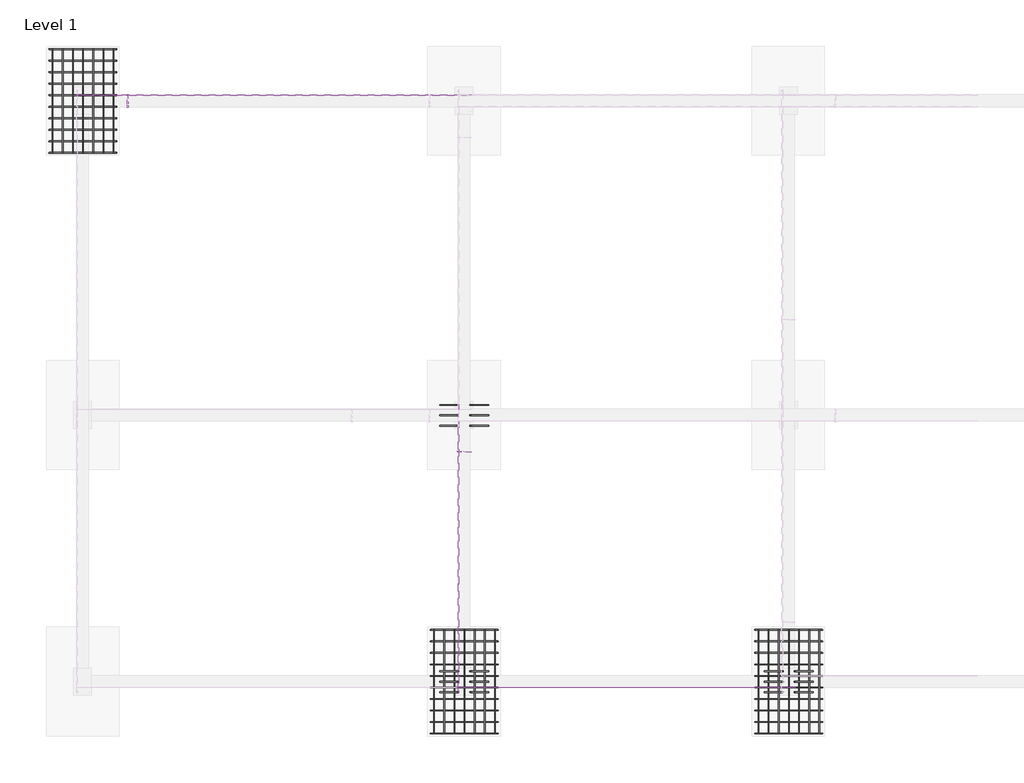
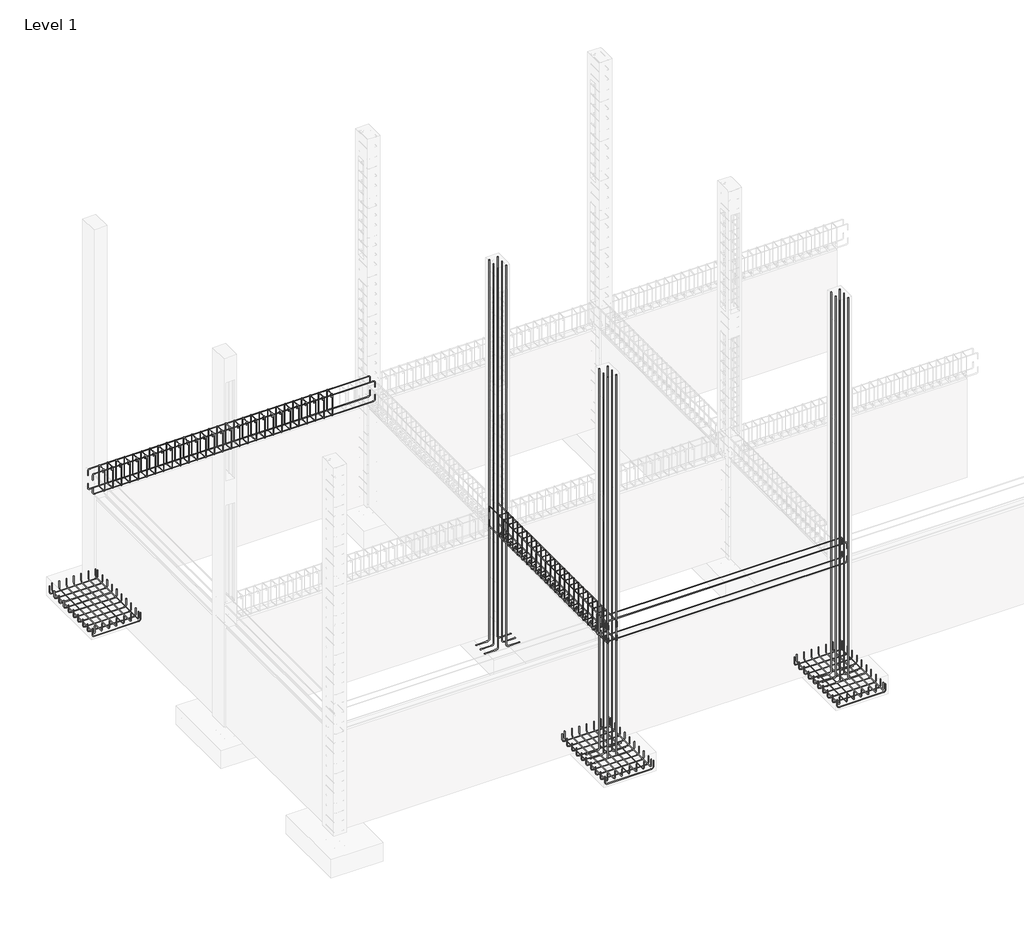
# One storey, part 4 of 8: 20 reinforcing bars.
"""IFC4 building model written with IfcOpenShell, lengths in millimetres."""

from ifc_helpers import new_model, si_unit, point, frame, origin, place, context, project, spatial, polyline, circle_curve, trimmed, segment, composite_curve, source, transform, mapped, element, save
from ifc_brep_helpers import swept_disk

model = new_model("IFC4")

# Units and contexts
model_context = context("Model", 3, world=origin())
ifc_project = project(units=[si_unit("LENGTHUNIT", "METRE", prefix="MILLI")], contexts=[model_context])

# Site, building, storey
site = spatial("IfcSite", under=ifc_project)
building = spatial("IfcBuilding", under=site)
storey = spatial("IfcBuildingStorey", under=building, Name="Level 1", Elevation=0.0)

# Reinforcing bars
placement = place(None, origin())
reinforcing_bar_shape = source(origin(), model_context, "Body", "SolidModel", [
    swept_disk(composite_curve([segment(polyline([(-8807.3422157, 3219.1306965, 2643.0183362), (-8807.3422157, 3219.1306965, 2528.7183362)]), True, "CONTINUOUS"), segment(trimmed(circle_curve(frame((-8841.8862157, 3219.1306965, 2528.7183362), z_axis=(0.0, 1.0, 0.0), x_axis=(34.54399999999987, 0.0, 0.0)), 34.544), [point((-8807.3422157, 3219.1306965, 2528.7183362))], [point((-8841.8862157, 3219.1306965, 2494.1743362))], True, "CARTESIAN"), True, "CONTINUOUS"), segment(polyline([(-8841.8862157, 3219.1306965, 2494.1743362), (-14435.2471545, 3219.1306965, 2494.1743362)]), True, "CONTINUOUS"), segment(trimmed(circle_curve(frame((-14435.2471545, 3219.1306965, 2528.7183362), z_axis=(0.0, 1.0, 0.0), x_axis=(0.0, 0.0, -34.54399999999987)), 34.544), [point((-14435.2471545, 3219.1306965, 2494.1743362))], [point((-14469.7911545, 3219.1306965, 2528.7183362))], True, "CARTESIAN"), True, "CONTINUOUS"), segment(polyline([(-14469.7911545, 3219.1306965, 2528.7183362), (-14469.7911545, 3219.1306965, 2643.0183362)]), True, "CONTINUOUS")], self_intersect=False), 5.969),
])
element("IfcReinforcingBar", 1, at=placement, inside=storey, context=model_context, shape_type="MappedRepresentation", body=[
    mapped(reinforcing_bar_shape, transform((0.0, 0.0, 0.0), x_axis=(1.0, 0.0, 0.0), y_axis=(0.0, 1.0, 0.0), z_axis=(0.0, 0.0, 1.0))),
    mapped(reinforcing_bar_shape, transform((0.0, -193.2513276, 0.0), x_axis=(1.0, 0.0, 0.0), y_axis=(0.0, 1.0, 0.0), z_axis=(0.0, 0.0, 1.0))),
])
reinforcing_bar_2_shape = source(origin(), model_context, "Body", "SolidModel", [
    swept_disk(composite_curve([segment(polyline([(-14469.7911545, 3219.1306965, 2843.3816638), (-14469.7911545, 3219.1306965, 2957.6816638)]), True, "CONTINUOUS"), segment(trimmed(circle_curve(frame((-14435.2471545, 3219.1306965, 2957.6816638), z_axis=(0.0, 1.0, 0.0), x_axis=(-34.54399999999987, 0.0, 0.0)), 34.544), [point((-14469.7911545, 3219.1306965, 2957.6816638))], [point((-14435.2471545, 3219.1306965, 2992.2256638))], True, "CARTESIAN"), True, "CONTINUOUS"), segment(polyline([(-14435.2471545, 3219.1306965, 2992.2256638), (-8841.8862157, 3219.1306965, 2992.2256638)]), True, "CONTINUOUS"), segment(trimmed(circle_curve(frame((-8841.8862157, 3219.1306965, 2957.6816638), z_axis=(0.0, 1.0, 0.0), x_axis=(0.0, 0.0, 34.54399999999987)), 34.544), [point((-8841.8862157, 3219.1306965, 2992.2256638))], [point((-8807.3422157, 3219.1306965, 2957.6816638))], True, "CARTESIAN"), True, "CONTINUOUS"), segment(polyline([(-8807.3422157, 3219.1306965, 2957.6816638), (-8807.3422157, 3219.1306965, 2843.3816638)]), True, "CONTINUOUS")], self_intersect=False), 5.969),
])
element("IfcReinforcingBar", 2, at=placement, inside=storey, context=model_context, shape_type="MappedRepresentation", body=[
    mapped(reinforcing_bar_2_shape, transform((0.0, 0.0, 0.0), x_axis=(1.0, 0.0, 0.0), y_axis=(0.0, 1.0, 0.0), z_axis=(0.0, 0.0, 1.0))),
    mapped(reinforcing_bar_2_shape, transform((0.0, -193.2513276, 0.0), x_axis=(1.0, 0.0, 0.0), y_axis=(0.0, 1.0, 0.0), z_axis=(0.0, 0.0, 1.0))),
])
reinforcing_bar_3_shape = source(origin(), model_context, "Body", "SolidModel", [
    swept_disk(composite_curve([segment(polyline([(-14263.0351545, 7767.9070829, 9105.9), (-14263.0351545, 7767.9070829, -307.9115)]), True, "CONTINUOUS"), segment(trimmed(circle_curve(frame((-14216.9341545, 7767.9070829, -307.9115), z_axis=(0.0, -1.0, 0.0), x_axis=(-46.10099999999875, 0.0, 0.0)), 46.101), [point((-14263.0351545, 7767.9070829, -307.9115))], [point((-14216.9341545, 7767.9070829, -354.0125))], True, "CARTESIAN"), True, "CONTINUOUS"), segment(polyline([(-14216.9341545, 7767.9070829, -354.0125), (-13950.3611545, 7767.9070829, -354.0125)]), True, "CONTINUOUS")], self_intersect=False), 8.001),
])
element("IfcReinforcingBar", 3, at=placement, inside=storey, context=model_context, shape_type="MappedRepresentation", body=[
    mapped(reinforcing_bar_3_shape, transform((0.0, 0.0, 0.0), x_axis=(1.0, 0.0, 0.0), y_axis=(0.0, 1.0, 0.0), z_axis=(0.0, 0.0, 1.0))),
    mapped(reinforcing_bar_3_shape, transform((0.0, -174.625, 0.0), x_axis=(1.0, 0.0, 0.0), y_axis=(0.0, 1.0, 0.0), z_axis=(0.0, 0.0, 1.0))),
    mapped(reinforcing_bar_3_shape, transform((0.0, -349.25, 0.0), x_axis=(1.0, 0.0, 0.0), y_axis=(0.0, 1.0, 0.0), z_axis=(0.0, 0.0, 1.0))),
])
reinforcing_bar_4_shape = source(origin(), model_context, "Body", "SolidModel", [
    swept_disk(composite_curve([segment(polyline([(-14772.5591545, 7767.9070829, -354.0125), (-14505.9861545, 7767.9070829, -354.0125)]), True, "CONTINUOUS"), segment(trimmed(circle_curve(frame((-14505.9861545, 7767.9070829, -307.9115), z_axis=(0.0, -1.0, 0.0), x_axis=(0.0, 0.0, -46.101)), 46.101), [point((-14505.9861545, 7767.9070829, -354.0125))], [point((-14459.8851545, 7767.9070829, -307.9115))], True, "CARTESIAN"), True, "CONTINUOUS"), segment(polyline([(-14459.8851545, 7767.9070829, -307.9115), (-14459.8851545, 7767.9070829, 9105.9)]), True, "CONTINUOUS")], self_intersect=False), 8.001),
])
element("IfcReinforcingBar", 4, at=placement, inside=storey, context=model_context, shape_type="MappedRepresentation", body=[
    mapped(reinforcing_bar_4_shape, transform((0.0, 0.0, 0.0), x_axis=(1.0, 0.0, 0.0), y_axis=(0.0, 1.0, 0.0), z_axis=(0.0, 0.0, 1.0))),
    mapped(reinforcing_bar_4_shape, transform((0.0, -174.625, 0.0), x_axis=(1.0, 0.0, 0.0), y_axis=(0.0, 1.0, 0.0), z_axis=(0.0, 0.0, 1.0))),
    mapped(reinforcing_bar_4_shape, transform((0.0, -349.25, 0.0), x_axis=(1.0, 0.0, 0.0), y_axis=(0.0, 1.0, 0.0), z_axis=(0.0, 0.0, 1.0))),
])
reinforcing_bar_5_shape = source(origin(), model_context, "Body", "SolidModel", [
    swept_disk(composite_curve([segment(polyline([(-14263.0351545, 3297.1300327, 9105.9), (-14263.0351545, 3297.1300327, -307.9115)]), True, "CONTINUOUS"), segment(trimmed(circle_curve(frame((-14216.9341545, 3297.1300327, -307.9115), z_axis=(0.0, -1.0, 0.0), x_axis=(-46.10099999999875, 0.0, 0.0)), 46.101), [point((-14263.0351545, 3297.1300327, -307.9115))], [point((-14216.9341545, 3297.1300327, -354.0125))], True, "CARTESIAN"), True, "CONTINUOUS"), segment(polyline([(-14216.9341545, 3297.1300327, -354.0125), (-13950.3611545, 3297.1300327, -354.0125)]), True, "CONTINUOUS")], self_intersect=False), 8.001),
])
element("IfcReinforcingBar", 5, at=placement, inside=storey, context=model_context, shape_type="MappedRepresentation", body=[
    mapped(reinforcing_bar_5_shape, transform((0.0, 0.0, 0.0), x_axis=(1.0, 0.0, 0.0), y_axis=(0.0, 1.0, 0.0), z_axis=(0.0, 0.0, 1.0))),
    mapped(reinforcing_bar_5_shape, transform((0.0, -174.625, 0.0), x_axis=(1.0, 0.0, 0.0), y_axis=(0.0, 1.0, 0.0), z_axis=(0.0, 0.0, 1.0))),
    mapped(reinforcing_bar_5_shape, transform((0.0, -349.25, 0.0), x_axis=(1.0, 0.0, 0.0), y_axis=(0.0, 1.0, 0.0), z_axis=(0.0, 0.0, 1.0))),
])
reinforcing_bar_6_shape = source(origin(), model_context, "Body", "SolidModel", [
    swept_disk(composite_curve([segment(polyline([(-14772.5591545, 3297.1300327, -354.0125), (-14505.9861545, 3297.1300327, -354.0125)]), True, "CONTINUOUS"), segment(trimmed(circle_curve(frame((-14505.9861545, 3297.1300327, -307.9115), z_axis=(0.0, -1.0, 0.0), x_axis=(0.0, 0.0, -46.101)), 46.101), [point((-14505.9861545, 3297.1300327, -354.0125))], [point((-14459.8851545, 3297.1300327, -307.9115))], True, "CARTESIAN"), True, "CONTINUOUS"), segment(polyline([(-14459.8851545, 3297.1300327, -307.9115), (-14459.8851545, 3297.1300327, 9105.9)]), True, "CONTINUOUS")], self_intersect=False), 8.001),
])
element("IfcReinforcingBar", 6, at=placement, inside=storey, context=model_context, shape_type="MappedRepresentation", body=[
    mapped(reinforcing_bar_6_shape, transform((0.0, 0.0, 0.0), x_axis=(1.0, 0.0, 0.0), y_axis=(0.0, 1.0, 0.0), z_axis=(0.0, 0.0, 1.0))),
    mapped(reinforcing_bar_6_shape, transform((0.0, -174.625, 0.0), x_axis=(1.0, 0.0, 0.0), y_axis=(0.0, 1.0, 0.0), z_axis=(0.0, 0.0, 1.0))),
    mapped(reinforcing_bar_6_shape, transform((0.0, -349.25, 0.0), x_axis=(1.0, 0.0, 0.0), y_axis=(0.0, 1.0, 0.0), z_axis=(0.0, 0.0, 1.0))),
])
reinforcing_bar_7_shape = source(origin(), model_context, "Body", "SolidModel", [
    swept_disk(composite_curve([segment(polyline([(-8817.2482157, 3297.1300327, 9105.9), (-8817.2482157, 3297.1300327, -307.9115)]), True, "CONTINUOUS"), segment(trimmed(circle_curve(frame((-8771.1472157, 3297.1300327, -307.9115), z_axis=(0.0, -1.0, 0.0), x_axis=(-46.10099999999875, 0.0, 0.0)), 46.101), [point((-8817.2482157, 3297.1300327, -307.9115))], [point((-8771.1472157, 3297.1300327, -354.0125))], True, "CARTESIAN"), True, "CONTINUOUS"), segment(polyline([(-8771.1472157, 3297.1300327, -354.0125), (-8504.5742157, 3297.1300327, -354.0125)]), True, "CONTINUOUS")], self_intersect=False), 8.001),
])
element("IfcReinforcingBar", 7, at=placement, inside=storey, context=model_context, shape_type="MappedRepresentation", body=[
    mapped(reinforcing_bar_7_shape, transform((0.0, 0.0, 0.0), x_axis=(1.0, 0.0, 0.0), y_axis=(0.0, 1.0, 0.0), z_axis=(0.0, 0.0, 1.0))),
    mapped(reinforcing_bar_7_shape, transform((0.0, -174.625, 0.0), x_axis=(1.0, 0.0, 0.0), y_axis=(0.0, 1.0, 0.0), z_axis=(0.0, 0.0, 1.0))),
    mapped(reinforcing_bar_7_shape, transform((0.0, -349.25, 0.0), x_axis=(1.0, 0.0, 0.0), y_axis=(0.0, 1.0, 0.0), z_axis=(0.0, 0.0, 1.0))),
])
reinforcing_bar_8_shape = source(origin(), model_context, "Body", "SolidModel", [
    swept_disk(composite_curve([segment(polyline([(-9326.7722157, 3297.1300327, -354.0125), (-9060.1992157, 3297.1300327, -354.0125)]), True, "CONTINUOUS"), segment(trimmed(circle_curve(frame((-9060.1992157, 3297.1300327, -307.9115), z_axis=(0.0, -1.0, 0.0), x_axis=(0.0, 0.0, -46.101)), 46.101), [point((-9060.1992157, 3297.1300327, -354.0125))], [point((-9014.0982157, 3297.1300327, -307.9115))], True, "CARTESIAN"), True, "CONTINUOUS"), segment(polyline([(-9014.0982157, 3297.1300327, -307.9115), (-9014.0982157, 3297.1300327, 9105.9)]), True, "CONTINUOUS")], self_intersect=False), 8.001),
])
element("IfcReinforcingBar", 8, at=placement, inside=storey, context=model_context, shape_type="MappedRepresentation", body=[
    mapped(reinforcing_bar_8_shape, transform((0.0, 0.0, 0.0), x_axis=(1.0, 0.0, 0.0), y_axis=(0.0, 1.0, 0.0), z_axis=(0.0, 0.0, 1.0))),
    mapped(reinforcing_bar_8_shape, transform((0.0, -174.625, 0.0), x_axis=(1.0, 0.0, 0.0), y_axis=(0.0, 1.0, 0.0), z_axis=(0.0, 0.0, 1.0))),
    mapped(reinforcing_bar_8_shape, transform((0.0, -349.25, 0.0), x_axis=(1.0, 0.0, 0.0), y_axis=(0.0, 1.0, 0.0), z_axis=(0.0, 0.0, 1.0))),
])
reinforcing_bar_9_shape = source(origin(), model_context, "Body", "SolidModel", [
    swept_disk(composite_curve([segment(polyline([(-20200.6033089, 13741.9865262, -216.662), (-20200.6033089, 13741.9865262, -369.062)]), True, "CONTINUOUS"), segment(trimmed(circle_curve(frame((-20244.6723089, 13741.9865262, -369.062), z_axis=(0.0, 1.0, 0.0), x_axis=(44.068999999999505, 0.0, 0.0)), 44.069), [point((-20200.6033089, 13741.9865262, -369.062))], [point((-20244.6723089, 13741.9865262, -413.131))], True, "CARTESIAN"), True, "CONTINUOUS"), segment(polyline([(-20244.6723089, 13741.9865262, -413.131), (-21287.5963089, 13741.9865262, -413.131)]), True, "CONTINUOUS"), segment(trimmed(circle_curve(frame((-21287.5963089, 13741.9865262, -369.062), z_axis=(0.0, 1.0, 0.0), x_axis=(0.0, 0.0, -44.06899999999996)), 44.069), [point((-21287.5963089, 13741.9865262, -413.131))], [point((-21331.6653089, 13741.9865262, -369.062))], True, "CARTESIAN"), True, "CONTINUOUS"), segment(polyline([(-21331.6653089, 13741.9865262, -369.062), (-21331.6653089, 13741.9865262, -216.662)]), True, "CONTINUOUS")], self_intersect=False), 5.969),
])
element("IfcReinforcingBar", 9, at=placement, inside=storey, context=model_context, shape_type="MappedRepresentation", body=[
    mapped(reinforcing_bar_9_shape, transform((0.0, 0.0, 0.0), x_axis=(1.0, 0.0, 0.0), y_axis=(0.0, 1.0, 0.0), z_axis=(0.0, 0.0, 1.0))),
    mapped(reinforcing_bar_9_shape, transform((0.0, -193.4068889, 0.0), x_axis=(1.0, 0.0, 0.0), y_axis=(0.0, 1.0, 0.0), z_axis=(0.0, 0.0, 1.0))),
    mapped(reinforcing_bar_9_shape, transform((0.0, -386.8137778, 0.0), x_axis=(1.0, 0.0, 0.0), y_axis=(0.0, 1.0, 0.0), z_axis=(0.0, 0.0, 1.0))),
    mapped(reinforcing_bar_9_shape, transform((0.0, -580.2206667, 0.0), x_axis=(1.0, 0.0, 0.0), y_axis=(0.0, 1.0, 0.0), z_axis=(0.0, 0.0, 1.0))),
    mapped(reinforcing_bar_9_shape, transform((0.0, -773.6275556, 0.0), x_axis=(1.0, 0.0, 0.0), y_axis=(0.0, 1.0, 0.0), z_axis=(0.0, 0.0, 1.0))),
    mapped(reinforcing_bar_9_shape, transform((0.0, -967.0344444, 0.0), x_axis=(1.0, 0.0, 0.0), y_axis=(0.0, 1.0, 0.0), z_axis=(0.0, 0.0, 1.0))),
    mapped(reinforcing_bar_9_shape, transform((0.0, -1160.4413333, 0.0), x_axis=(1.0, 0.0, 0.0), y_axis=(0.0, 1.0, 0.0), z_axis=(0.0, 0.0, 1.0))),
    mapped(reinforcing_bar_9_shape, transform((0.0, -1353.8482222, 0.0), x_axis=(1.0, 0.0, 0.0), y_axis=(0.0, 1.0, 0.0), z_axis=(0.0, 0.0, 1.0))),
    mapped(reinforcing_bar_9_shape, transform((0.0, -1547.2551111, 0.0), x_axis=(1.0, 0.0, 0.0), y_axis=(0.0, 1.0, 0.0), z_axis=(0.0, 0.0, 1.0))),
    mapped(reinforcing_bar_9_shape, transform((0.0, -1740.662, 0.0), x_axis=(1.0, 0.0, 0.0), y_axis=(0.0, 1.0, 0.0), z_axis=(0.0, 0.0, 1.0))),
])
reinforcing_bar_10_shape = source(origin(), model_context, "Body", "SolidModel", [
    swept_disk(composite_curve([segment(polyline([(-21274.1343089, 13741.9865262, -165.481), (-21274.1343089, 13741.9865262, -317.881)]), True, "CONTINUOUS"), segment(trimmed(circle_curve(frame((-21274.1343089, 13697.9175262, -317.881), z_axis=(-1.0, 0.0, 0.0), x_axis=(0.0, 44.068999999999505, 0.0)), 44.069), [point((-21274.1343089, 13741.9865262, -317.881))], [point((-21274.1343089, 13697.9175262, -361.95))], True, "CARTESIAN"), True, "CONTINUOUS"), segment(polyline([(-21274.1343089, 13697.9175262, -361.95), (-21274.1343089, 12045.3935262, -361.95)]), True, "CONTINUOUS"), segment(trimmed(circle_curve(frame((-21274.1343089, 12045.3935262, -317.881), z_axis=(-1.0, 0.0, 0.0), x_axis=(0.0, 0.0, -44.06900000000002)), 44.069), [point((-21274.1343089, 12045.3935262, -361.95))], [point((-21274.1343089, 12001.3245262, -317.881))], True, "CARTESIAN"), True, "CONTINUOUS"), segment(polyline([(-21274.1343089, 12001.3245262, -317.881), (-21274.1343089, 12001.3245262, -165.481)]), True, "CONTINUOUS")], self_intersect=False), 5.969),
])
element("IfcReinforcingBar", 10, at=placement, inside=storey, context=model_context, shape_type="MappedRepresentation", body=[
    mapped(reinforcing_bar_10_shape, transform((0.0, 0.0, 0.0), x_axis=(1.0, 0.0, 0.0), y_axis=(0.0, 1.0, 0.0), z_axis=(0.0, 0.0, 1.0))),
    mapped(reinforcing_bar_10_shape, transform((170.5954914, 0.0, 0.0), x_axis=(1.0, 0.0, 0.0), y_axis=(0.0, 1.0, 0.0), z_axis=(0.0, 0.0, 1.0))),
    mapped(reinforcing_bar_10_shape, transform((341.1909829, 0.0, 0.0), x_axis=(1.0, 0.0, 0.0), y_axis=(0.0, 1.0, 0.0), z_axis=(0.0, 0.0, 1.0))),
    mapped(reinforcing_bar_10_shape, transform((511.7864743, 0.0, 0.0), x_axis=(1.0, 0.0, 0.0), y_axis=(0.0, 1.0, 0.0), z_axis=(0.0, 0.0, 1.0))),
    mapped(reinforcing_bar_10_shape, transform((682.3819658, 0.0, 0.0), x_axis=(1.0, 0.0, 0.0), y_axis=(0.0, 1.0, 0.0), z_axis=(0.0, 0.0, 1.0))),
    mapped(reinforcing_bar_10_shape, transform((852.9774572, 0.0, 0.0), x_axis=(1.0, 0.0, 0.0), y_axis=(0.0, 1.0, 0.0), z_axis=(0.0, 0.0, 1.0))),
    mapped(reinforcing_bar_10_shape, transform((1023.5729487, 0.0, 0.0), x_axis=(1.0, 0.0, 0.0), y_axis=(0.0, 1.0, 0.0), z_axis=(0.0, 0.0, 1.0))),
])
reinforcing_bar_11_shape = source(origin(), model_context, "Body", "SolidModel", [
    swept_disk(composite_curve([segment(polyline([(-13795.9291545, 3992.8360327, -216.662), (-13795.9291545, 3992.8360327, -369.062)]), True, "CONTINUOUS"), segment(trimmed(circle_curve(frame((-13839.9981545, 3992.8360327, -369.062), z_axis=(0.0, 1.0, 0.0), x_axis=(44.068999999999505, 0.0, 0.0)), 44.069), [point((-13795.9291545, 3992.8360327, -369.062))], [point((-13839.9981545, 3992.8360327, -413.131))], True, "CARTESIAN"), True, "CONTINUOUS"), segment(polyline([(-13839.9981545, 3992.8360327, -413.131), (-14882.9221545, 3992.8360327, -413.131)]), True, "CONTINUOUS"), segment(trimmed(circle_curve(frame((-14882.9221545, 3992.8360327, -369.062), z_axis=(0.0, 1.0, 0.0), x_axis=(0.0, 0.0, -44.06899999999996)), 44.069), [point((-14882.9221545, 3992.8360327, -413.131))], [point((-14926.9911545, 3992.8360327, -369.062))], True, "CARTESIAN"), True, "CONTINUOUS"), segment(polyline([(-14926.9911545, 3992.8360327, -369.062), (-14926.9911545, 3992.8360327, -216.662)]), True, "CONTINUOUS")], self_intersect=False), 5.969),
])
element("IfcReinforcingBar", 11, at=placement, inside=storey, context=model_context, shape_type="MappedRepresentation", body=[
    mapped(reinforcing_bar_11_shape, transform((0.0, 0.0, 0.0), x_axis=(1.0, 0.0, 0.0), y_axis=(0.0, 1.0, 0.0), z_axis=(0.0, 0.0, 1.0))),
    mapped(reinforcing_bar_11_shape, transform((0.0, -193.4068889, 0.0), x_axis=(1.0, 0.0, 0.0), y_axis=(0.0, 1.0, 0.0), z_axis=(0.0, 0.0, 1.0))),
    mapped(reinforcing_bar_11_shape, transform((0.0, -386.8137778, 0.0), x_axis=(1.0, 0.0, 0.0), y_axis=(0.0, 1.0, 0.0), z_axis=(0.0, 0.0, 1.0))),
    mapped(reinforcing_bar_11_shape, transform((0.0, -580.2206667, 0.0), x_axis=(1.0, 0.0, 0.0), y_axis=(0.0, 1.0, 0.0), z_axis=(0.0, 0.0, 1.0))),
    mapped(reinforcing_bar_11_shape, transform((0.0, -773.6275556, 0.0), x_axis=(1.0, 0.0, 0.0), y_axis=(0.0, 1.0, 0.0), z_axis=(0.0, 0.0, 1.0))),
    mapped(reinforcing_bar_11_shape, transform((0.0, -967.0344444, 0.0), x_axis=(1.0, 0.0, 0.0), y_axis=(0.0, 1.0, 0.0), z_axis=(0.0, 0.0, 1.0))),
    mapped(reinforcing_bar_11_shape, transform((0.0, -1160.4413333, 0.0), x_axis=(1.0, 0.0, 0.0), y_axis=(0.0, 1.0, 0.0), z_axis=(0.0, 0.0, 1.0))),
    mapped(reinforcing_bar_11_shape, transform((0.0, -1353.8482222, 0.0), x_axis=(1.0, 0.0, 0.0), y_axis=(0.0, 1.0, 0.0), z_axis=(0.0, 0.0, 1.0))),
    mapped(reinforcing_bar_11_shape, transform((0.0, -1547.2551111, 0.0), x_axis=(1.0, 0.0, 0.0), y_axis=(0.0, 1.0, 0.0), z_axis=(0.0, 0.0, 1.0))),
    mapped(reinforcing_bar_11_shape, transform((0.0, -1740.662, 0.0), x_axis=(1.0, 0.0, 0.0), y_axis=(0.0, 1.0, 0.0), z_axis=(0.0, 0.0, 1.0))),
])
reinforcing_bar_12_shape = source(origin(), model_context, "Body", "SolidModel", [
    swept_disk(composite_curve([segment(polyline([(-14869.4601545, 3992.8360327, -165.481), (-14869.4601545, 3992.8360327, -317.881)]), True, "CONTINUOUS"), segment(trimmed(circle_curve(frame((-14869.4601545, 3948.7670327, -317.881), z_axis=(-1.0, 0.0, 0.0), x_axis=(0.0, 44.06899999999996, 0.0)), 44.069), [point((-14869.4601545, 3992.8360327, -317.881))], [point((-14869.4601545, 3948.7670327, -361.95))], True, "CARTESIAN"), True, "CONTINUOUS"), segment(polyline([(-14869.4601545, 3948.7670327, -361.95), (-14869.4601545, 2296.2430327, -361.95)]), True, "CONTINUOUS"), segment(trimmed(circle_curve(frame((-14869.4601545, 2296.2430327, -317.881), z_axis=(-1.0, 0.0, 0.0), x_axis=(0.0, 0.0, -44.06900000000002)), 44.069), [point((-14869.4601545, 2296.2430327, -361.95))], [point((-14869.4601545, 2252.1740327, -317.881))], True, "CARTESIAN"), True, "CONTINUOUS"), segment(polyline([(-14869.4601545, 2252.1740327, -317.881), (-14869.4601545, 2252.1740327, -165.481)]), True, "CONTINUOUS")], self_intersect=False), 5.969),
])
element("IfcReinforcingBar", 12, at=placement, inside=storey, context=model_context, shape_type="MappedRepresentation", body=[
    mapped(reinforcing_bar_12_shape, transform((0.0, 0.0, 0.0), x_axis=(1.0, 0.0, 0.0), y_axis=(0.0, 1.0, 0.0), z_axis=(0.0, 0.0, 1.0))),
    mapped(reinforcing_bar_12_shape, transform((170.5954914, 0.0, 0.0), x_axis=(1.0, 0.0, 0.0), y_axis=(0.0, 1.0, 0.0), z_axis=(0.0, 0.0, 1.0))),
    mapped(reinforcing_bar_12_shape, transform((341.1909829, 0.0, 0.0), x_axis=(1.0, 0.0, 0.0), y_axis=(0.0, 1.0, 0.0), z_axis=(0.0, 0.0, 1.0))),
    mapped(reinforcing_bar_12_shape, transform((511.7864743, 0.0, 0.0), x_axis=(1.0, 0.0, 0.0), y_axis=(0.0, 1.0, 0.0), z_axis=(0.0, 0.0, 1.0))),
    mapped(reinforcing_bar_12_shape, transform((682.3819658, 0.0, 0.0), x_axis=(1.0, 0.0, 0.0), y_axis=(0.0, 1.0, 0.0), z_axis=(0.0, 0.0, 1.0))),
    mapped(reinforcing_bar_12_shape, transform((852.9774572, 0.0, 0.0), x_axis=(1.0, 0.0, 0.0), y_axis=(0.0, 1.0, 0.0), z_axis=(0.0, 0.0, 1.0))),
    mapped(reinforcing_bar_12_shape, transform((1023.5729487, 0.0, 0.0), x_axis=(1.0, 0.0, 0.0), y_axis=(0.0, 1.0, 0.0), z_axis=(0.0, 0.0, 1.0))),
])
reinforcing_bar_13_shape = source(origin(), model_context, "Body", "SolidModel", [
    swept_disk(composite_curve([segment(polyline([(-8350.1422157, 3992.8360327, -216.662), (-8350.1422157, 3992.8360327, -369.062)]), True, "CONTINUOUS"), segment(trimmed(circle_curve(frame((-8394.2112157, 3992.8360327, -369.062), z_axis=(0.0, 1.0, 0.0), x_axis=(44.068999999999505, 0.0, 0.0)), 44.069), [point((-8350.1422157, 3992.8360327, -369.062))], [point((-8394.2112157, 3992.8360327, -413.131))], True, "CARTESIAN"), True, "CONTINUOUS"), segment(polyline([(-8394.2112157, 3992.8360327, -413.131), (-9437.1352157, 3992.8360327, -413.131)]), True, "CONTINUOUS"), segment(trimmed(circle_curve(frame((-9437.1352157, 3992.8360327, -369.062), z_axis=(0.0, 1.0, 0.0), x_axis=(0.0, 0.0, -44.06899999999996)), 44.069), [point((-9437.1352157, 3992.8360327, -413.131))], [point((-9481.2042157, 3992.8360327, -369.062))], True, "CARTESIAN"), True, "CONTINUOUS"), segment(polyline([(-9481.2042157, 3992.8360327, -369.062), (-9481.2042157, 3992.8360327, -216.662)]), True, "CONTINUOUS")], self_intersect=False), 5.969),
])
element("IfcReinforcingBar", 13, at=placement, inside=storey, context=model_context, shape_type="MappedRepresentation", body=[
    mapped(reinforcing_bar_13_shape, transform((0.0, 0.0, 0.0), x_axis=(1.0, 0.0, 0.0), y_axis=(0.0, 1.0, 0.0), z_axis=(0.0, 0.0, 1.0))),
    mapped(reinforcing_bar_13_shape, transform((0.0, -193.4068889, 0.0), x_axis=(1.0, 0.0, 0.0), y_axis=(0.0, 1.0, 0.0), z_axis=(0.0, 0.0, 1.0))),
    mapped(reinforcing_bar_13_shape, transform((0.0, -386.8137778, 0.0), x_axis=(1.0, 0.0, 0.0), y_axis=(0.0, 1.0, 0.0), z_axis=(0.0, 0.0, 1.0))),
    mapped(reinforcing_bar_13_shape, transform((0.0, -580.2206667, 0.0), x_axis=(1.0, 0.0, 0.0), y_axis=(0.0, 1.0, 0.0), z_axis=(0.0, 0.0, 1.0))),
    mapped(reinforcing_bar_13_shape, transform((0.0, -773.6275556, 0.0), x_axis=(1.0, 0.0, 0.0), y_axis=(0.0, 1.0, 0.0), z_axis=(0.0, 0.0, 1.0))),
    mapped(reinforcing_bar_13_shape, transform((0.0, -967.0344444, 0.0), x_axis=(1.0, 0.0, 0.0), y_axis=(0.0, 1.0, 0.0), z_axis=(0.0, 0.0, 1.0))),
    mapped(reinforcing_bar_13_shape, transform((0.0, -1160.4413333, 0.0), x_axis=(1.0, 0.0, 0.0), y_axis=(0.0, 1.0, 0.0), z_axis=(0.0, 0.0, 1.0))),
    mapped(reinforcing_bar_13_shape, transform((0.0, -1353.8482222, 0.0), x_axis=(1.0, 0.0, 0.0), y_axis=(0.0, 1.0, 0.0), z_axis=(0.0, 0.0, 1.0))),
    mapped(reinforcing_bar_13_shape, transform((0.0, -1547.2551111, 0.0), x_axis=(1.0, 0.0, 0.0), y_axis=(0.0, 1.0, 0.0), z_axis=(0.0, 0.0, 1.0))),
    mapped(reinforcing_bar_13_shape, transform((0.0, -1740.662, 0.0), x_axis=(1.0, 0.0, 0.0), y_axis=(0.0, 1.0, 0.0), z_axis=(0.0, 0.0, 1.0))),
])
reinforcing_bar_14_shape = source(origin(), model_context, "Body", "SolidModel", [
    swept_disk(composite_curve([segment(polyline([(-9423.6732157, 3992.8360327, -165.481), (-9423.6732157, 3992.8360327, -317.881)]), True, "CONTINUOUS"), segment(trimmed(circle_curve(frame((-9423.6732157, 3948.7670327, -317.881), z_axis=(-1.0, 0.0, 0.0), x_axis=(0.0, 44.06899999999996, 0.0)), 44.069), [point((-9423.6732157, 3992.8360327, -317.881))], [point((-9423.6732157, 3948.7670327, -361.95))], True, "CARTESIAN"), True, "CONTINUOUS"), segment(polyline([(-9423.6732157, 3948.7670327, -361.95), (-9423.6732157, 2296.2430327, -361.95)]), True, "CONTINUOUS"), segment(trimmed(circle_curve(frame((-9423.6732157, 2296.2430327, -317.881), z_axis=(-1.0, 0.0, 0.0), x_axis=(0.0, 0.0, -44.06900000000002)), 44.069), [point((-9423.6732157, 2296.2430327, -361.95))], [point((-9423.6732157, 2252.1740327, -317.881))], True, "CARTESIAN"), True, "CONTINUOUS"), segment(polyline([(-9423.6732157, 2252.1740327, -317.881), (-9423.6732157, 2252.1740327, -165.481)]), True, "CONTINUOUS")], self_intersect=False), 5.969),
])
element("IfcReinforcingBar", 14, at=placement, inside=storey, context=model_context, shape_type="MappedRepresentation", body=[
    mapped(reinforcing_bar_14_shape, transform((0.0, 0.0, 0.0), x_axis=(1.0, 0.0, 0.0), y_axis=(0.0, 1.0, 0.0), z_axis=(0.0, 0.0, 1.0))),
    mapped(reinforcing_bar_14_shape, transform((170.5954914, 0.0, 0.0), x_axis=(1.0, 0.0, 0.0), y_axis=(0.0, 1.0, 0.0), z_axis=(0.0, 0.0, 1.0))),
    mapped(reinforcing_bar_14_shape, transform((341.1909829, 0.0, 0.0), x_axis=(1.0, 0.0, 0.0), y_axis=(0.0, 1.0, 0.0), z_axis=(0.0, 0.0, 1.0))),
    mapped(reinforcing_bar_14_shape, transform((511.7864743, 0.0, 0.0), x_axis=(1.0, 0.0, 0.0), y_axis=(0.0, 1.0, 0.0), z_axis=(0.0, 0.0, 1.0))),
    mapped(reinforcing_bar_14_shape, transform((682.3819658, 0.0, 0.0), x_axis=(1.0, 0.0, 0.0), y_axis=(0.0, 1.0, 0.0), z_axis=(0.0, 0.0, 1.0))),
    mapped(reinforcing_bar_14_shape, transform((852.9774572, 0.0, 0.0), x_axis=(1.0, 0.0, 0.0), y_axis=(0.0, 1.0, 0.0), z_axis=(0.0, 0.0, 1.0))),
    mapped(reinforcing_bar_14_shape, transform((1023.5729487, 0.0, 0.0), x_axis=(1.0, 0.0, 0.0), y_axis=(0.0, 1.0, 0.0), z_axis=(0.0, 0.0, 1.0))),
])
reinforcing_bar_15_shape = source(origin(), model_context, "Body", "SolidModel", [
    swept_disk(composite_curve([segment(polyline([(-20874.4653089, 12775.0298624, 2643.0183362), (-20874.4653089, 12775.0298624, 2528.7183362)]), True, "CONTINUOUS"), segment(trimmed(circle_curve(frame((-20839.9213089, 12775.0298624, 2528.7183362), z_axis=(0.0, -1.0, 0.0), x_axis=(-34.54399999999805, 0.0, 0.0)), 34.544), [point((-20874.4653089, 12775.0298624, 2528.7183362))], [point((-20839.9213089, 12775.0298624, 2494.1743362))], True, "CARTESIAN"), True, "CONTINUOUS"), segment(polyline([(-20839.9213089, 12775.0298624, 2494.1743362), (-14287.6731545, 12775.0298624, 2494.1743362)]), True, "CONTINUOUS"), segment(trimmed(circle_curve(frame((-14287.6731545, 12775.0298624, 2528.7183362), z_axis=(0.0, -1.0, 0.0), x_axis=(0.0, 0.0, -34.54399999999987)), 34.544), [point((-14287.6731545, 12775.0298624, 2494.1743362))], [point((-14253.1291545, 12775.0298624, 2528.7183362))], True, "CARTESIAN"), True, "CONTINUOUS"), segment(polyline([(-14253.1291545, 12775.0298624, 2528.7183362), (-14253.1291545, 12775.0298624, 2643.0183362)]), True, "CONTINUOUS")], self_intersect=False), 5.969),
])
element("IfcReinforcingBar", 15, at=placement, inside=storey, context=model_context, shape_type="MappedRepresentation", body=[
    mapped(reinforcing_bar_15_shape, transform((0.0, 0.0, 0.0), x_axis=(1.0, 0.0, 0.0), y_axis=(0.0, 1.0, 0.0), z_axis=(0.0, 0.0, 1.0))),
    mapped(reinforcing_bar_15_shape, transform((0.0, 193.2513276, 0.0), x_axis=(1.0, 0.0, 0.0), y_axis=(0.0, 1.0, 0.0), z_axis=(0.0, 0.0, 1.0))),
])
reinforcing_bar_16_shape = source(origin(), model_context, "Body", "SolidModel", [
    swept_disk(composite_curve([segment(polyline([(-14253.1291545, 12775.0298624, 2843.3816638), (-14253.1291545, 12775.0298624, 2957.6816638)]), True, "CONTINUOUS"), segment(trimmed(circle_curve(frame((-14287.6731545, 12775.0298624, 2957.6816638), z_axis=(0.0, -1.0, 0.0), x_axis=(34.54399999999987, 0.0, 0.0)), 34.544), [point((-14253.1291545, 12775.0298624, 2957.6816638))], [point((-14287.6731545, 12775.0298624, 2992.2256638))], True, "CARTESIAN"), True, "CONTINUOUS"), segment(polyline([(-14287.6731545, 12775.0298624, 2992.2256638), (-20839.9213089, 12775.0298624, 2992.2256638)]), True, "CONTINUOUS"), segment(trimmed(circle_curve(frame((-20839.9213089, 12775.0298624, 2957.6816638), z_axis=(0.0, -1.0, 0.0), x_axis=(0.0, 0.0, 34.54399999999987)), 34.544), [point((-20839.9213089, 12775.0298624, 2992.2256638))], [point((-20874.4653089, 12775.0298624, 2957.6816638))], True, "CARTESIAN"), True, "CONTINUOUS"), segment(polyline([(-20874.4653089, 12775.0298624, 2957.6816638), (-20874.4653089, 12775.0298624, 2843.3816638)]), True, "CONTINUOUS")], self_intersect=False), 5.969),
])
element("IfcReinforcingBar", 16, at=placement, inside=storey, context=model_context, shape_type="MappedRepresentation", body=[
    mapped(reinforcing_bar_16_shape, transform((0.0, 0.0, 0.0), x_axis=(1.0, 0.0, 0.0), y_axis=(0.0, 1.0, 0.0), z_axis=(0.0, 0.0, 1.0))),
    mapped(reinforcing_bar_16_shape, transform((0.0, 193.2513276, 0.0), x_axis=(1.0, 0.0, 0.0), y_axis=(0.0, 1.0, 0.0), z_axis=(0.0, 0.0, 1.0))),
])
reinforcing_bar_17_shape = source(origin(), model_context, "Body", "SolidModel", [
    swept_disk(composite_curve([segment(polyline([(-15262.6578092, 12824.8894597, 2909.8575394), (-15262.6578092, 12768.0252626, 2966.7217364)]), True, "CONTINUOUS"), segment(trimmed(circle_curve(frame((-15262.6578092, 12784.2795262, 2982.976), z_axis=(-1.0, 0.0, 0.0), x_axis=(0.0, -16.25426359999983, -16.254263600000286)), 22.987), [point((-15262.6578092, 12768.0252626, 2966.7217364))], [point((-15262.6578092, 12784.2795262, 3005.963))], True, "CARTESIAN"), True, "CONTINUOUS"), segment(polyline([(-15262.6578092, 12784.2795262, 3005.963), (-15262.6578092, 12959.0315262, 3005.963)]), True, "CONTINUOUS"), segment(trimmed(circle_curve(frame((-15262.6578092, 12959.0315262, 2982.976), z_axis=(-1.0, 0.0, 0.0), x_axis=(0.0, 0.0, 22.98700000000008)), 22.987), [point((-15262.6578092, 12959.0315262, 3005.963))], [point((-15262.6578092, 12982.0185262, 2982.976))], True, "CARTESIAN"), True, "CONTINUOUS"), segment(polyline([(-15262.6578092, 12982.0185262, 2982.976), (-15262.6578092, 12982.0185262, 2503.424)]), True, "CONTINUOUS"), segment(trimmed(circle_curve(frame((-15261.8383109, 12959.0461386, 2503.424), z_axis=(-0.9993643184948482, -0.03565051078634927, 0.0), x_axis=(-0.8194982999993954, 22.97238759999891, 0.0)), 22.987), [point((-15262.6578092, 12982.0185262, 2503.424))], [point((-15261.8383109, 12959.0461386, 2480.437))], True, "CARTESIAN"), True, "CONTINUOUS"), segment(polyline([(-15261.8383109, 12959.0461386, 2480.437), (-15255.6033075, 12784.2649138, 2480.437)]), True, "CONTINUOUS"), segment(trimmed(circle_curve(frame((-15255.6033075, 12784.2649138, 2503.424), z_axis=(-0.9993643184948482, -0.03565051078634927, 0.0), x_axis=(0.0, 0.0, -22.98700000000008)), 22.987), [point((-15255.6033075, 12784.2649138, 2480.437))], [point((-15254.7838092, 12761.2925262, 2503.424))], True, "CARTESIAN"), True, "CONTINUOUS"), segment(polyline([(-15254.7838092, 12761.2925262, 2503.424), (-15254.7838092, 12761.2925262, 2982.976)]), True, "CONTINUOUS"), segment(trimmed(circle_curve(frame((-15254.7838092, 12784.2795262, 2982.976), z_axis=(-1.0, 0.0, 0.0), x_axis=(0.0, -22.98699999999917, 0.0)), 22.987), [point((-15254.7838092, 12761.2925262, 2982.976))], [point((-15254.7838092, 12800.5337898, 2999.2302636))], True, "CARTESIAN"), True, "CONTINUOUS"), segment(polyline([(-15254.7838092, 12800.5337898, 2999.2302636), (-15254.7838092, 12857.3979868, 2942.3660665)]), True, "CONTINUOUS")], self_intersect=False), 3.937),
])
element("IfcReinforcingBar", 17, at=placement, inside=storey, context=model_context, shape_type="MappedRepresentation", body=[
    mapped(reinforcing_bar_17_shape, transform((0.0, 0.0, 0.0), x_axis=(1.0, 0.0, 0.0), y_axis=(0.0, 1.0, 0.0), z_axis=(0.0, 0.0, 1.0))),
    mapped(reinforcing_bar_17_shape, transform((-198.0422037, 0.0, 0.0), x_axis=(1.0, 0.0, 0.0), y_axis=(0.0, 1.0, 0.0), z_axis=(0.0, 0.0, 1.0))),
    mapped(reinforcing_bar_17_shape, transform((-396.0844074, 0.0, 0.0), x_axis=(1.0, 0.0, 0.0), y_axis=(0.0, 1.0, 0.0), z_axis=(0.0, 0.0, 1.0))),
    mapped(reinforcing_bar_17_shape, transform((-594.1266111, 0.0, 0.0), x_axis=(1.0, 0.0, 0.0), y_axis=(0.0, 1.0, 0.0), z_axis=(0.0, 0.0, 1.0))),
    mapped(reinforcing_bar_17_shape, transform((-792.1688148, 0.0, 0.0), x_axis=(1.0, 0.0, 0.0), y_axis=(0.0, 1.0, 0.0), z_axis=(0.0, 0.0, 1.0))),
    mapped(reinforcing_bar_17_shape, transform((-990.2110185, 0.0, 0.0), x_axis=(1.0, 0.0, 0.0), y_axis=(0.0, 1.0, 0.0), z_axis=(0.0, 0.0, 1.0))),
    mapped(reinforcing_bar_17_shape, transform((-1188.2532221, 0.0, 0.0), x_axis=(1.0, 0.0, 0.0), y_axis=(0.0, 1.0, 0.0), z_axis=(0.0, 0.0, 1.0))),
    mapped(reinforcing_bar_17_shape, transform((-1386.2954258, 0.0, 0.0), x_axis=(1.0, 0.0, 0.0), y_axis=(0.0, 1.0, 0.0), z_axis=(0.0, 0.0, 1.0))),
    mapped(reinforcing_bar_17_shape, transform((-1584.3376295, 0.0, 0.0), x_axis=(1.0, 0.0, 0.0), y_axis=(0.0, 1.0, 0.0), z_axis=(0.0, 0.0, 1.0))),
    mapped(reinforcing_bar_17_shape, transform((-1782.3798332, 0.0, 0.0), x_axis=(1.0, 0.0, 0.0), y_axis=(0.0, 1.0, 0.0), z_axis=(0.0, 0.0, 1.0))),
    mapped(reinforcing_bar_17_shape, transform((-1980.4220369, 0.0, 0.0), x_axis=(1.0, 0.0, 0.0), y_axis=(0.0, 1.0, 0.0), z_axis=(0.0, 0.0, 1.0))),
    mapped(reinforcing_bar_17_shape, transform((-2178.4642406, 0.0, 0.0), x_axis=(1.0, 0.0, 0.0), y_axis=(0.0, 1.0, 0.0), z_axis=(0.0, 0.0, 1.0))),
    mapped(reinforcing_bar_17_shape, transform((-2376.5064443, 0.0, 0.0), x_axis=(1.0, 0.0, 0.0), y_axis=(0.0, 1.0, 0.0), z_axis=(0.0, 0.0, 1.0))),
    mapped(reinforcing_bar_17_shape, transform((-2574.548648, 0.0, 0.0), x_axis=(1.0, 0.0, 0.0), y_axis=(0.0, 1.0, 0.0), z_axis=(0.0, 0.0, 1.0))),
    mapped(reinforcing_bar_17_shape, transform((-2772.5908517, 0.0, 0.0), x_axis=(1.0, 0.0, 0.0), y_axis=(0.0, 1.0, 0.0), z_axis=(0.0, 0.0, 1.0))),
    mapped(reinforcing_bar_17_shape, transform((-2970.6330554, 0.0, 0.0), x_axis=(1.0, 0.0, 0.0), y_axis=(0.0, 1.0, 0.0), z_axis=(0.0, 0.0, 1.0))),
    mapped(reinforcing_bar_17_shape, transform((-3168.6752591, 0.0, 0.0), x_axis=(1.0, 0.0, 0.0), y_axis=(0.0, 1.0, 0.0), z_axis=(0.0, 0.0, 1.0))),
    mapped(reinforcing_bar_17_shape, transform((-3366.7174628, 0.0, 0.0), x_axis=(1.0, 0.0, 0.0), y_axis=(0.0, 1.0, 0.0), z_axis=(0.0, 0.0, 1.0))),
    mapped(reinforcing_bar_17_shape, transform((-3564.7596664, 0.0, 0.0), x_axis=(1.0, 0.0, 0.0), y_axis=(0.0, 1.0, 0.0), z_axis=(0.0, 0.0, 1.0))),
    mapped(reinforcing_bar_17_shape, transform((-3762.8018701, 0.0, 0.0), x_axis=(1.0, 0.0, 0.0), y_axis=(0.0, 1.0, 0.0), z_axis=(0.0, 0.0, 1.0))),
    mapped(reinforcing_bar_17_shape, transform((-3960.8440738, 0.0, 0.0), x_axis=(1.0, 0.0, 0.0), y_axis=(0.0, 1.0, 0.0), z_axis=(0.0, 0.0, 1.0))),
    mapped(reinforcing_bar_17_shape, transform((-4158.8862775, 0.0, 0.0), x_axis=(1.0, 0.0, 0.0), y_axis=(0.0, 1.0, 0.0), z_axis=(0.0, 0.0, 1.0))),
    mapped(reinforcing_bar_17_shape, transform((-4356.9284812, 0.0, 0.0), x_axis=(1.0, 0.0, 0.0), y_axis=(0.0, 1.0, 0.0), z_axis=(0.0, 0.0, 1.0))),
    mapped(reinforcing_bar_17_shape, transform((-4554.9706849, 0.0, 0.0), x_axis=(1.0, 0.0, 0.0), y_axis=(0.0, 1.0, 0.0), z_axis=(0.0, 0.0, 1.0))),
    mapped(reinforcing_bar_17_shape, transform((-4753.0128886, 0.0, 0.0), x_axis=(1.0, 0.0, 0.0), y_axis=(0.0, 1.0, 0.0), z_axis=(0.0, 0.0, 1.0))),
    mapped(reinforcing_bar_17_shape, transform((-4951.0550923, 0.0, 0.0), x_axis=(1.0, 0.0, 0.0), y_axis=(0.0, 1.0, 0.0), z_axis=(0.0, 0.0, 1.0))),
    mapped(reinforcing_bar_17_shape, transform((-5149.097296, 0.0, 0.0), x_axis=(1.0, 0.0, 0.0), y_axis=(0.0, 1.0, 0.0), z_axis=(0.0, 0.0, 1.0))),
    mapped(reinforcing_bar_17_shape, transform((-5347.1394997, 0.0, 0.0), x_axis=(1.0, 0.0, 0.0), y_axis=(0.0, 1.0, 0.0), z_axis=(0.0, 0.0, 1.0))),
])
reinforcing_bar_18_shape = source(origin(), model_context, "Body", "SolidModel", [
    swept_disk(composite_curve([segment(polyline([(-14458.0858183, 7777.8130829, 2643.0183362), (-14458.0858183, 7777.8130829, 2528.7183362)]), True, "CONTINUOUS"), segment(trimmed(circle_curve(frame((-14458.0858183, 7743.2690829, 2528.7183362), z_axis=(-1.0, 0.0, 0.0), x_axis=(0.0, 34.54399999999987, 0.0)), 34.544), [point((-14458.0858183, 7777.8130829, 2528.7183362))], [point((-14458.0858183, 7743.2690829, 2494.1743362))], True, "CARTESIAN"), True, "CONTINUOUS"), segment(polyline([(-14458.0858183, 7743.2690829, 2494.1743362), (-14458.0858183, 2972.5180327, 2494.1743362)]), True, "CONTINUOUS"), segment(trimmed(circle_curve(frame((-14458.0858183, 2972.5180327, 2528.7183362), z_axis=(-1.0, 0.0, 0.0), x_axis=(0.0, 0.0, -34.54399999999987)), 34.544), [point((-14458.0858183, 2972.5180327, 2494.1743362))], [point((-14458.0858183, 2937.9740327, 2528.7183362))], True, "CARTESIAN"), True, "CONTINUOUS"), segment(polyline([(-14458.0858183, 2937.9740327, 2528.7183362), (-14458.0858183, 2937.9740327, 2643.0183362)]), True, "CONTINUOUS")], self_intersect=False), 5.969),
])
element("IfcReinforcingBar", 18, at=placement, inside=storey, context=model_context, shape_type="MappedRepresentation", body=[
    mapped(reinforcing_bar_18_shape, transform((0.0, 0.0, 0.0), x_axis=(1.0, 0.0, 0.0), y_axis=(0.0, 1.0, 0.0), z_axis=(0.0, 0.0, 1.0))),
    mapped(reinforcing_bar_18_shape, transform((204.9566638, 0.0, 0.0), x_axis=(1.0, 0.0, 0.0), y_axis=(0.0, 1.0, 0.0), z_axis=(0.0, 0.0, 1.0))),
])
reinforcing_bar_19_shape = source(origin(), model_context, "Body", "SolidModel", [
    swept_disk(composite_curve([segment(polyline([(-14458.0858183, 2937.9740327, 2843.3816638), (-14458.0858183, 2937.9740327, 2957.6816638)]), True, "CONTINUOUS"), segment(trimmed(circle_curve(frame((-14458.0858183, 2972.5180327, 2957.6816638), z_axis=(-1.0, 0.0, 0.0), x_axis=(0.0, -34.54399999999987, 0.0)), 34.544), [point((-14458.0858183, 2937.9740327, 2957.6816638))], [point((-14458.0858183, 2972.5180327, 2992.2256638))], True, "CARTESIAN"), True, "CONTINUOUS"), segment(polyline([(-14458.0858183, 2972.5180327, 2992.2256638), (-14458.0858183, 7743.2690829, 2992.2256638)]), True, "CONTINUOUS"), segment(trimmed(circle_curve(frame((-14458.0858183, 7743.2690829, 2957.6816638), z_axis=(-1.0, 0.0, 0.0), x_axis=(0.0, 0.0, 34.54399999999987)), 34.544), [point((-14458.0858183, 7743.2690829, 2992.2256638))], [point((-14458.0858183, 7777.8130829, 2957.6816638))], True, "CARTESIAN"), True, "CONTINUOUS"), segment(polyline([(-14458.0858183, 7777.8130829, 2957.6816638), (-14458.0858183, 7777.8130829, 2843.3816638)]), True, "CONTINUOUS")], self_intersect=False), 5.969),
])
element("IfcReinforcingBar", 19, at=placement, inside=storey, context=model_context, shape_type="MappedRepresentation", body=[
    mapped(reinforcing_bar_19_shape, transform((0.0, 0.0, 0.0), x_axis=(1.0, 0.0, 0.0), y_axis=(0.0, 1.0, 0.0), z_axis=(0.0, 0.0, 1.0))),
    mapped(reinforcing_bar_19_shape, transform((204.9566638, 0.0, 0.0), x_axis=(1.0, 0.0, 0.0), y_axis=(0.0, 1.0, 0.0), z_axis=(0.0, 0.0, 1.0))),
])
reinforcing_bar_20_shape = source(origin(), model_context, "Body", "SolidModel", [
    swept_disk(composite_curve([segment(polyline([(-14408.226221, 7360.7450829, 2576.5424606), (-14465.0904181, 7360.7450829, 2519.6782636)]), True, "CONTINUOUS"), segment(trimmed(circle_curve(frame((-14448.8361545, 7360.7450829, 2503.424), z_axis=(0.0, -1.0, 0.0), x_axis=(-16.25426359999983, 0.0, 16.25426359999983)), 22.987), [point((-14465.0904181, 7360.7450829, 2519.6782636))], [point((-14448.8361545, 7360.7450829, 2480.437))], True, "CARTESIAN"), True, "CONTINUOUS"), segment(polyline([(-14448.8361545, 7360.7450829, 2480.437), (-14274.0841545, 7360.7450829, 2480.437)]), True, "CONTINUOUS"), segment(trimmed(circle_curve(frame((-14274.0841545, 7360.7450829, 2503.424), z_axis=(0.0, -1.0, 0.0), x_axis=(0.0, 0.0, -22.98700000000008)), 22.987), [point((-14274.0841545, 7360.7450829, 2480.437))], [point((-14251.0971545, 7360.7450829, 2503.424))], True, "CARTESIAN"), True, "CONTINUOUS"), segment(polyline([(-14251.0971545, 7360.7450829, 2503.424), (-14251.0971545, 7360.7450829, 2982.976)]), True, "CONTINUOUS"), segment(trimmed(circle_curve(frame((-14274.0695421, 7361.5645812, 2982.976), z_axis=(-0.03565051078635315, -0.9993643184948481, 0.0), x_axis=(22.97238760000073, -0.8194983000003049, 0.0)), 22.987), [point((-14251.0971545, 7360.7450829, 2982.976))], [point((-14274.0695421, 7361.5645812, 3005.963))], True, "CARTESIAN"), True, "CONTINUOUS"), segment(polyline([(-14274.0695421, 7361.5645812, 3005.963), (-14448.8507669, 7367.7995846, 3005.963)]), True, "CONTINUOUS"), segment(trimmed(circle_curve(frame((-14448.8507669, 7367.7995846, 2982.976), z_axis=(-0.03565051078635315, -0.9993643184948481, 0.0), x_axis=(0.0, 0.0, 22.98700000000008)), 22.987), [point((-14448.8507669, 7367.7995846, 3005.963))], [point((-14471.8231545, 7368.6190829, 2982.976))], True, "CARTESIAN"), True, "CONTINUOUS"), segment(polyline([(-14471.8231545, 7368.6190829, 2982.976), (-14471.8231545, 7368.6190829, 2503.424)]), True, "CONTINUOUS"), segment(trimmed(circle_curve(frame((-14448.8361545, 7368.6190829, 2503.424), z_axis=(0.0, -1.0, 0.0), x_axis=(-22.98699999999917, 0.0, 0.0)), 22.987), [point((-14471.8231545, 7368.6190829, 2503.424))], [point((-14432.5818909, 7368.6190829, 2487.1697364))], True, "CARTESIAN"), True, "CONTINUOUS"), segment(polyline([(-14432.5818909, 7368.6190829, 2487.1697364), (-14375.7176938, 7368.6190829, 2544.0339335)]), True, "CONTINUOUS")], self_intersect=False), 3.937),
])
element("IfcReinforcingBar", 20, at=placement, inside=storey, context=model_context, shape_type="MappedRepresentation", body=[
    mapped(reinforcing_bar_20_shape, transform((0.0, 0.0, 0.0), x_axis=(1.0, 0.0, 0.0), y_axis=(0.0, 1.0, 0.0), z_axis=(0.0, 0.0, 1.0))),
    mapped(reinforcing_bar_20_shape, transform((0.0, -190.7477643, 0.0), x_axis=(1.0, 0.0, 0.0), y_axis=(0.0, 1.0, 0.0), z_axis=(0.0, 0.0, 1.0))),
    mapped(reinforcing_bar_20_shape, transform((0.0, -381.4955286, 0.0), x_axis=(1.0, 0.0, 0.0), y_axis=(0.0, 1.0, 0.0), z_axis=(0.0, 0.0, 1.0))),
    mapped(reinforcing_bar_20_shape, transform((0.0, -572.2432929, 0.0), x_axis=(1.0, 0.0, 0.0), y_axis=(0.0, 1.0, 0.0), z_axis=(0.0, 0.0, 1.0))),
    mapped(reinforcing_bar_20_shape, transform((0.0, -762.9910572, 0.0), x_axis=(1.0, 0.0, 0.0), y_axis=(0.0, 1.0, 0.0), z_axis=(0.0, 0.0, 1.0))),
    mapped(reinforcing_bar_20_shape, transform((0.0, -953.7388215, 0.0), x_axis=(1.0, 0.0, 0.0), y_axis=(0.0, 1.0, 0.0), z_axis=(0.0, 0.0, 1.0))),
    mapped(reinforcing_bar_20_shape, transform((0.0, -1144.4865858, 0.0), x_axis=(1.0, 0.0, 0.0), y_axis=(0.0, 1.0, 0.0), z_axis=(0.0, 0.0, 1.0))),
    mapped(reinforcing_bar_20_shape, transform((0.0, -1335.2343501, 0.0), x_axis=(1.0, 0.0, 0.0), y_axis=(0.0, 1.0, 0.0), z_axis=(0.0, 0.0, 1.0))),
    mapped(reinforcing_bar_20_shape, transform((0.0, -1525.9821143, 0.0), x_axis=(1.0, 0.0, 0.0), y_axis=(0.0, 1.0, 0.0), z_axis=(0.0, 0.0, 1.0))),
    mapped(reinforcing_bar_20_shape, transform((0.0, -1716.7298786, 0.0), x_axis=(1.0, 0.0, 0.0), y_axis=(0.0, 1.0, 0.0), z_axis=(0.0, 0.0, 1.0))),
    mapped(reinforcing_bar_20_shape, transform((0.0, -1907.4776429, 0.0), x_axis=(1.0, 0.0, 0.0), y_axis=(0.0, 1.0, 0.0), z_axis=(0.0, 0.0, 1.0))),
    mapped(reinforcing_bar_20_shape, transform((0.0, -2098.2254072, 0.0), x_axis=(1.0, 0.0, 0.0), y_axis=(0.0, 1.0, 0.0), z_axis=(0.0, 0.0, 1.0))),
    mapped(reinforcing_bar_20_shape, transform((0.0, -2288.9731715, 0.0), x_axis=(1.0, 0.0, 0.0), y_axis=(0.0, 1.0, 0.0), z_axis=(0.0, 0.0, 1.0))),
    mapped(reinforcing_bar_20_shape, transform((0.0, -2479.7209358, 0.0), x_axis=(1.0, 0.0, 0.0), y_axis=(0.0, 1.0, 0.0), z_axis=(0.0, 0.0, 1.0))),
    mapped(reinforcing_bar_20_shape, transform((0.0, -2670.4687001, 0.0), x_axis=(1.0, 0.0, 0.0), y_axis=(0.0, 1.0, 0.0), z_axis=(0.0, 0.0, 1.0))),
    mapped(reinforcing_bar_20_shape, transform((0.0, -2861.2164644, 0.0), x_axis=(1.0, 0.0, 0.0), y_axis=(0.0, 1.0, 0.0), z_axis=(0.0, 0.0, 1.0))),
    mapped(reinforcing_bar_20_shape, transform((0.0, -3051.9642287, 0.0), x_axis=(1.0, 0.0, 0.0), y_axis=(0.0, 1.0, 0.0), z_axis=(0.0, 0.0, 1.0))),
    mapped(reinforcing_bar_20_shape, transform((0.0, -3242.711993, 0.0), x_axis=(1.0, 0.0, 0.0), y_axis=(0.0, 1.0, 0.0), z_axis=(0.0, 0.0, 1.0))),
    mapped(reinforcing_bar_20_shape, transform((0.0, -3433.4597573, 0.0), x_axis=(1.0, 0.0, 0.0), y_axis=(0.0, 1.0, 0.0), z_axis=(0.0, 0.0, 1.0))),
    mapped(reinforcing_bar_20_shape, transform((0.0, -3624.2075216, 0.0), x_axis=(1.0, 0.0, 0.0), y_axis=(0.0, 1.0, 0.0), z_axis=(0.0, 0.0, 1.0))),
    mapped(reinforcing_bar_20_shape, transform((0.0, -3814.9552859, 0.0), x_axis=(1.0, 0.0, 0.0), y_axis=(0.0, 1.0, 0.0), z_axis=(0.0, 0.0, 1.0))),
    mapped(reinforcing_bar_20_shape, transform((0.0, -4005.7030502, 0.0), x_axis=(1.0, 0.0, 0.0), y_axis=(0.0, 1.0, 0.0), z_axis=(0.0, 0.0, 1.0))),
])

save(model, "model.ifc")

# Revit data of these elements
# Elements 1, 2, 3, 4, 5, 6, 7, 8, 9, 10, 11, 12, 13, 14, 15, 16, 17, 18, 19, 20 (IfcReinforcingBar)
#   Phase Created = New Construction
